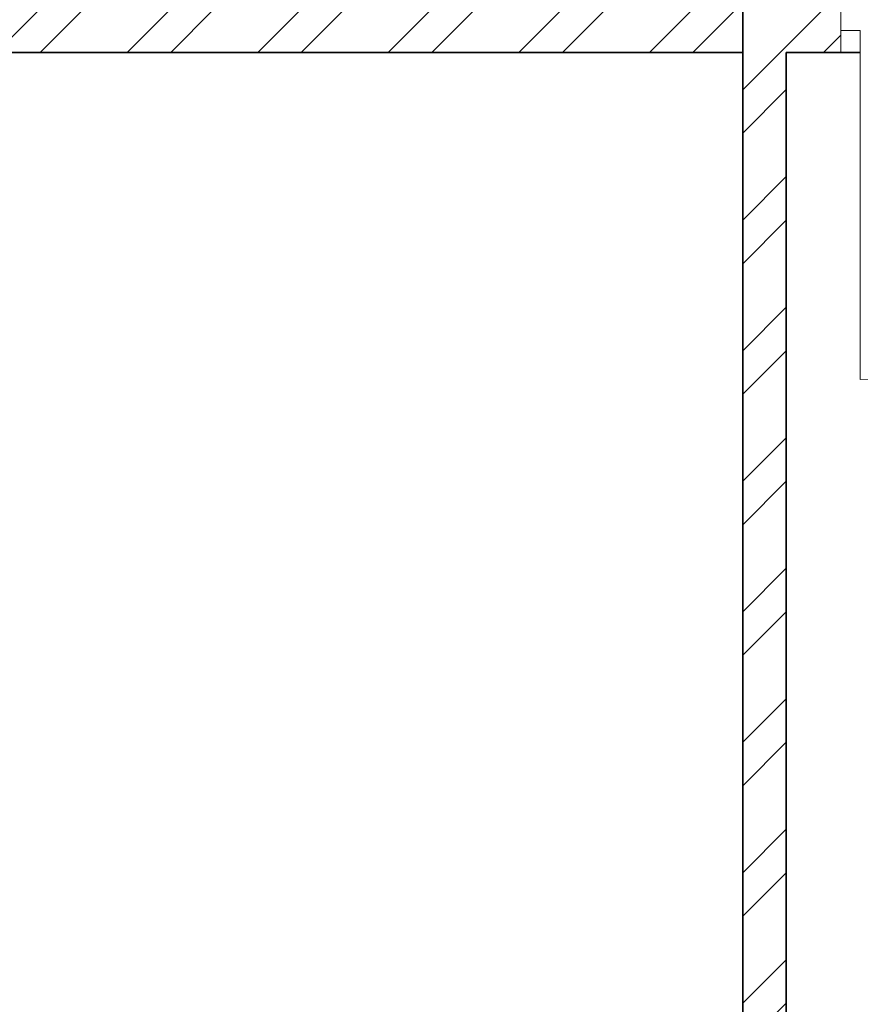
# Model space of a CAD drawing. Units: inches. Extents: x 1962 to 2771, y 1245 to 2660.
# Tile 31 of 114: x 2160 to 2247, y 1831 to 1932. Entities that reach past the tile are written whole.
import ezdxf

# ---------------------------------------------------------------- set-up
doc = ezdxf.new("R2010")
doc.units = ezdxf.units.IN
for name, color, linetype, lineweight in [('A-DOOR', 3, 'Continuous', 18), ('A-WALL', 7, 'Continuous', 35), ('A-WALL-PATT', 252, 'Continuous', 13)]:
    doc.layers.add(name, color=color, linetype=linetype, lineweight=lineweight)

msp = doc.modelspace()

# ---------------------------------------------------------------- hatches: boundary and pattern name
at = {"layer": 'A-WALL-PATT'}
h = msp.add_hatch(dxfattribs=at)
h.set_pattern_fill('ANSI32', color=256)
h.paths.add_polyline_path([(2090.8074, 2467.3437), (2141.6481, 2467.3437), (2141.6481, 2469.5937), (2141.6481, 2471.8437), (2086.3074, 2471.8437), (2086.3074, 2422.5333), (2090.8074, 2422.5333)])
h.paths.add_polyline_path([(2282.7664, 2471.8437), (2204.8982, 2471.8437), (2204.8982, 2467.3437), (2234.8074, 2467.3437), (2234.8074, 2311.3437), (2228.7492, 2311.3437), (2228.7492, 2306.8437), (2234.8074, 2306.8437), (2331.9227, 2306.8437), (2331.9227, 2309.0937), (2331.9227, 2311.3437), (2239.3074, 2311.3437), (2239.3074, 2467.3437), (2282.7664, 2467.3437), (2282.7664, 2469.5937)])
h.paths.add_polyline_path([(2471.4531, 2519.8437), (2552.011, 2519.8437), (2564.3996, 2519.8437), (2564.3996, 2511.1389), (2568.8996, 2511.1389), (2568.8996, 2524.3437), (2466.9531, 2524.3437), (2466.9531, 2471.8437), (2450.0749, 2471.8437), (2446.4672, 2471.8437), (2446.4672, 2467.3437), (2450.0749, 2467.3437), (2475.9988, 2467.3437), (2475.9988, 2469.5937), (2475.9988, 2471.8437), (2471.4531, 2471.8437)])
h.paths.add_polyline_path([(2575.2231, 2469.5937), (2575.2231, 2471.8437), (2568.8996, 2471.8437), (2568.8996, 2487.1389), (2564.3996, 2487.1389), (2564.3996, 2471.8437), (2556.511, 2471.8437), (2499.2904, 2471.8437), (2499.2904, 2467.3437), (2507.8074, 2467.3437), (2507.8074, 2311.3437), (2414.863, 2311.3437), (2414.863, 2306.8437), (2512.3074, 2306.8437), (2517.0114, 2306.8437), (2517.0114, 2309.0937), (2517.0114, 2311.3437), (2512.3074, 2311.3437), (2512.3074, 2467.3437), (2575.2231, 2467.3437)])
h.paths.add_polyline_path([(2660.8074, 2471.8437), (2600.9602, 2471.8437), (2600.9602, 2467.3437), (2656.3074, 2467.3437), (2656.3074, 2432.5704), (2660.8074, 2432.5704)])
h.paths.add_polyline_path([(2660.8074, 2372.5704), (2656.3074, 2372.5704), (2656.3074, 2311.3437), (2600.276, 2311.3437), (2600.276, 2309.0937), (2600.276, 2306.8437), (2656.3074, 2306.8437), (2656.3074, 2296.2593), (2660.8074, 2296.2593)])
h.paths.add_polyline_path([(2572.3074, 2306.8437), (2577.1385, 2306.8437), (2577.1385, 2311.3437), (2551.082, 2311.3437), (2551.082, 2306.8437), (2567.8074, 2306.8437), (2567.8074, 2258.8437), (2540.0574, 2258.8437), (2540.0574, 2256.5937), (2540.0574, 2254.3437), (2567.8074, 2254.3437), (2656.3074, 2254.3437), (2656.3074, 2236.9085), (2660.8074, 2236.9085), (2660.8074, 2272.2593), (2656.3074, 2272.2593), (2656.3074, 2258.8437), (2572.3074, 2258.8437)])
h.paths.add_polyline_path([(2512.3074, 2254.3437), (2518.8716, 2254.3437), (2518.8716, 2256.5937), (2518.8716, 2258.8437), (2507.8074, 2258.8437), (2507.8074, 2177.8437), (2567.8074, 2177.8437), (2567.8074, 2172.9628), (2572.3074, 2172.9628), (2572.3074, 2177.8437), (2656.3074, 2177.8437), (2656.3074, 2166.4846), (2660.8074, 2166.4846), (2660.8074, 2200.9085), (2656.3074, 2200.9085), (2656.3074, 2182.3437), (2512.3074, 2182.3437)])
h.paths.add_polyline_path([(2656.3074, 2129.8437), (2572.3074, 2129.8437), (2572.3074, 2150.3044), (2570.0574, 2150.3044), (2567.8074, 2150.3044), (2567.8074, 2129.8437), (2507.8074, 2129.8437), (2507.8074, 2116.3027), (2510.0574, 2116.3027), (2512.3074, 2116.3027), (2512.3074, 2125.3437), (2567.8074, 2125.3437), (2572.3074, 2125.3437), (2656.3074, 2125.3437)])
h.paths.add_polyline_path([(2090.8074, 2362.5333), (2086.3074, 2362.5333), (2086.3074, 2298.6242), (2090.8074, 2298.6242), (2090.8074, 2306.8437), (2174.8074, 2306.8437), (2174.8074, 2286.4178), (2179.3074, 2286.4178), (2179.3074, 2306.8437), (2192.8641, 2306.8437), (2192.8641, 2309.0937), (2192.8641, 2311.3437), (2090.8074, 2311.3437)])
h.paths.add_polyline_path([(2209.156, 2258.8437), (2179.3074, 2258.8437), (2179.3074, 2263.2236), (2177.0574, 2263.2236), (2174.8074, 2263.2236), (2174.8074, 2258.8437), (2090.8074, 2258.8437), (2090.8074, 2274.6242), (2086.3074, 2274.6242), (2086.3074, 2238.2967), (2088.5574, 2238.2967), (2090.8074, 2238.2967), (2090.8074, 2254.3437), (2209.156, 2254.3437)])
h.paths.add_polyline_path([(2090.8074, 2177.8437), (2234.8074, 2177.8437), (2234.8074, 2173.1428), (2239.3074, 2173.1428), (2239.3074, 2258.8437), (2230.8442, 2258.8437), (2230.8442, 2256.5937), (2230.8442, 2254.3437), (2234.8074, 2254.3437), (2234.8074, 2182.3437), (2090.8074, 2182.3437), (2090.8074, 2202.2967), (2086.3074, 2202.2967), (2086.3074, 2140.0389), (2090.8074, 2140.0389)])
h.paths.add_polyline_path([(2090.8074, 2080.0389), (2086.3074, 2080.0389), (2086.3074, 2033.8437), (2090.8074, 2033.8437)], flags=17)
h.paths.add_polyline_path([(2244.9405, 2033.8437), (2239.3074, 2033.8437), (2239.3074, 2142.0665), (2237.2592, 2142.0665), (2234.8074, 2142.0665), (2234.8074, 2033.8437), (2090.8074, 2033.8437), (2076.5204, 2033.8437), (2072.0204, 2033.8437), (2072.0204, 2000.4493), (2076.5204, 2000.4493), (2076.5204, 2029.3437), (2090.8074, 2029.3437), (2244.9405, 2029.3437), (2244.9405, 2031.5937)])
h.paths.add_polyline_path([(2234.8074, 1933.3437), (2076.5204, 1933.3437), (2076.5204, 1952.4493), (2074.2704, 1952.4493), (2072.0204, 1952.4493), (2072.0204, 1933.3437), (2072.0204, 1928.8437), (2234.8074, 1928.8437)])
h.paths.add_polyline_path([(2090.8074, 1928.8437), (2086.3074, 1928.8437), (2086.3074, 1906.5013), (2090.8074, 1906.5013)])
h.paths.add_polyline_path([(2090.8074, 1846.5013), (2086.3074, 1846.5013), (2086.3074, 1769.9917), (2088.5574, 1769.9917), (2090.8074, 1769.9917), (2090.8074, 1780.3437), (2234.8074, 1780.3437), (2234.8074, 1708.3437), (2230.3764, 1708.3437), (2230.3764, 1703.8437), (2239.3074, 1703.8437), (2239.3074, 1792.6669), (2237.0574, 1792.6669), (2234.8074, 1792.6669), (2234.8074, 1784.8437), (2090.8074, 1784.8437)])
h.paths.add_polyline_path([(2239.3074, 1928.8437), (2244.9405, 1928.8437), (2244.9405, 1931.0937), (2244.9405, 1933.3437), (2234.8074, 1933.3437), (2234.8074, 1928.8437), (2234.8074, 1825.5949), (2239.3074, 1825.5949)])
h.paths.add_polyline_path([(2148.0425, 1649.0937), (2148.0425, 1651.3437), (2090.8074, 1651.3437), (2090.8074, 1646.8437), (2148.0425, 1646.8437)], flags=0)
h.paths.add_polyline_path([(2207.5601, 1708.3437), (2090.8074, 1708.3437), (2090.8074, 1703.8437), (2174.8074, 1703.8437), (2174.8074, 1651.3437), (2170.4457, 1651.3437), (2170.4457, 1646.8437), (2195.9924, 1646.8437), (2195.9924, 1649.0937), (2195.9924, 1651.3437), (2179.3074, 1651.3437), (2179.3074, 1703.8437), (2207.5601, 1703.8437), (2207.5601, 1706.0937)])
h.paths.add_polyline_path([(2090.8074, 1733.9917), (2086.3074, 1733.9917), (2086.3074, 1696.1032), (2088.5574, 1696.1032), (2090.8074, 1696.1032)])
h.paths.add_polyline_path([(2090.8074, 1672.1032), (2086.3074, 1672.1032), (2086.3074, 1600.3335), (2090.8074, 1600.3335)])
h.paths.add_polyline_path([(2090.8074, 1540.3335), (2086.3074, 1540.3335), (2086.3074, 1486.3437), (2139.6766, 1486.3437), (2139.6766, 1490.8437), (2090.8074, 1490.8437)])
h.paths.add_polyline_path([(2302.3876, 1490.8437), (2239.3074, 1490.8437), (2239.3074, 1646.8437), (2335.9994, 1646.8437), (2335.9994, 1651.3437), (2229.884, 1651.3437), (2229.884, 1646.8437), (2234.8074, 1646.8437), (2234.8074, 1490.8437), (2202.7103, 1490.8437), (2202.7103, 1488.5937), (2202.7103, 1486.3437), (2275.0699, 1486.3437), (2275.0699, 1475.772), (2279.5699, 1475.772), (2279.5699, 1486.3437), (2302.3876, 1486.3437)])
h.paths.add_polyline_path([(2279.5699, 1451.772), (2275.0699, 1451.772), (2275.0699, 1438.3437), (2174.8074, 1438.3437), (2174.8074, 1486.3437), (2179.7922, 1486.3437), (2179.7922, 1490.8437), (2163.3585, 1490.8437), (2163.3585, 1488.5937), (2163.3585, 1486.3437), (2170.3074, 1486.3437), (2170.3074, 1433.8437), (2279.5699, 1433.8437)])
h.paths.add_polyline_path([(2427.2363, 1490.8437), (2375.8074, 1490.8437), (2375.8074, 1646.8437), (2381.6401, 1646.8437), (2381.6401, 1651.3437), (2365.887, 1651.3437), (2365.887, 1649.0937), (2365.887, 1646.8437), (2371.3074, 1646.8437), (2371.3074, 1490.8437), (2327.5627, 1490.8437), (2327.5627, 1488.5937), (2327.5627, 1486.3437), (2371.3074, 1486.3437), (2371.3074, 1433.8437), (2375.8074, 1433.8437), (2375.8074, 1486.3437), (2427.2363, 1486.3437)])
h.paths.add_polyline_path([(2512.3074, 1646.8437), (2519.4351, 1646.8437), (2519.4351, 1649.0937), (2519.4351, 1651.3437), (2507.8074, 1651.3437), (2416.0063, 1651.3437), (2416.0063, 1649.0937), (2416.0063, 1646.8437), (2507.8074, 1646.8437), (2507.8074, 1490.8437), (2497.0532, 1490.8437), (2497.0532, 1488.5937), (2497.0532, 1486.3437), (2574.9344, 1486.3437), (2574.9344, 1476.0181), (2579.4344, 1476.0181), (2579.4344, 1486.3437), (2584.4872, 1486.3437), (2584.3074, 1490.8437), (2512.3074, 1490.8437)])
h.paths.add_polyline_path([(2470.5091, 1486.3437), (2473.9767, 1486.3437), (2473.9767, 1490.8437), (2449.6605, 1490.8437), (2449.6605, 1488.5937), (2449.6605, 1486.3437), (2466.0091, 1486.3437), (2466.0091, 1433.8437), (2470.5091, 1433.8437), (2579.4344, 1433.8437), (2579.4344, 1452.0181), (2574.9344, 1452.0181), (2574.9344, 1438.3437), (2554.5091, 1438.3437), (2470.5091, 1438.3437)])
h.paths.add_polyline_path([(2656.3074, 1490.8437), (2611.86, 1490.8437), (2611.86, 1486.3437), (2656.3074, 1486.3437)])
h.paths.add_polyline_path([(2660.8074, 1532.7007), (2658.5574, 1532.7007), (2656.3074, 1532.7007), (2656.3074, 1486.3437), (2660.8074, 1486.3437)])
h.paths.add_polyline_path([(2660.8074, 1664.9663), (2656.3074, 1664.9663), (2656.3074, 1651.3437), (2602.2313, 1651.3437), (2602.2313, 1646.8437), (2656.3074, 1646.8437), (2656.3074, 1592.7007), (2660.8074, 1592.7007)])
h.paths.add_polyline_path([(2660.8074, 1724.5221), (2656.3074, 1724.5221), (2656.3074, 1703.8437), (2542.4725, 1703.8437), (2542.4725, 1699.3437), (2567.8074, 1699.3437), (2567.8074, 1651.3437), (2552.7766, 1651.3437), (2552.7766, 1649.0937), (2552.7766, 1646.8437), (2577.2878, 1646.8437), (2577.2878, 1649.0937), (2577.2878, 1651.3437), (2572.3074, 1651.3437), (2572.3074, 1699.3437), (2656.3074, 1699.3437), (2656.3074, 1688.9663), (2660.8074, 1688.9663)])
h.paths.add_polyline_path([(2660.8074, 1880.6524), (2656.3074, 1880.6524), (2656.3074, 1832.8437), (2512.3074, 1832.8437), (2512.3074, 1837.8959), (2507.8074, 1837.8959), (2507.8074, 1828.3437), (2567.8074, 1828.3437), (2567.8074, 1804.3437), (2572.3074, 1804.3437), (2572.3074, 1828.3437), (2656.3074, 1828.3437), (2656.3074, 1818.6778), (2660.8074, 1818.6778)])
h.paths.add_polyline_path([(2660.8074, 1794.6778), (2656.3074, 1794.6778), (2656.3074, 1780.3437), (2572.3074, 1780.3437), (2572.3074, 1783.0303), (2570.0574, 1783.0303), (2567.8074, 1783.0303), (2567.8074, 1780.3437), (2507.8074, 1780.3437), (2507.8074, 1699.3437), (2517.8858, 1699.3437), (2517.8858, 1701.5937), (2517.8858, 1703.8437), (2512.3074, 1703.8437), (2512.3074, 1775.8437), (2656.3074, 1775.8437), (2656.3074, 1760.5221), (2660.8074, 1760.5221)])
h.paths.add_polyline_path([(2660.8074, 1981.3437), (2660.8074, 2020.2808), (2658.5574, 2020.2808), (2656.3074, 2020.2808), (2656.3074, 1981.3437), (2512.3074, 1981.3437), (2512.3074, 2086.6996), (2507.8074, 2086.6996), (2507.8074, 1981.3437), (2375.8074, 1981.3437), (2375.8074, 1986.8505), (2373.5574, 1986.8505), (2371.3074, 1986.8505), (2371.3074, 1973.2607), (2375.8074, 1973.2607), (2375.8074, 1976.8437), (2507.8074, 1976.8437), (2507.8074, 1865.4281), (2510.0574, 1865.4281), (2512.3074, 1865.4281), (2512.3074, 1976.8437), (2660.8074, 1976.8437)])
h.paths.add_polyline_path([(2375.8074, 1940.297), (2373.5574, 1940.297), (2371.3074, 1940.297), (2371.3074, 1933.3437), (2278.4434, 1933.3437), (2278.4434, 1928.8437), (2371.3074, 1928.8437), (2371.3074, 1651.3437), (2375.8074, 1651.3437)])
h.paths.add_polyline_path([(2660.8074, 1976.8437), (2656.3074, 1976.8437), (2656.3074, 1940.6524), (2660.8074, 1940.6524)], flags=17)
h.paths.add_polyline_path([(2660.8074, 2142.4846), (2656.3074, 2142.4846), (2656.3074, 2080.2808), (2660.8074, 2080.2808)])
h.paths.add_polyline_path([(2381.4189, 2311.3437), (2375.8074, 2311.3437), (2375.8074, 2467.3437), (2424.7242, 2467.3437), (2424.7242, 2469.5937), (2424.7242, 2471.8437), (2375.8074, 2471.8437), (2375.8074, 2524.3437), (2371.3074, 2524.3437), (2371.3074, 2471.8437), (2307.2097, 2471.8437), (2307.2097, 2467.3437), (2371.3074, 2467.3437), (2371.3074, 2311.3437), (2366.8901, 2311.3437), (2366.8901, 2306.8437), (2371.3074, 2306.8437), (2371.3074, 2033.8437), (2279.6589, 2033.8437), (2279.6589, 2029.3437), (2371.3074, 2029.3437), (2371.3074, 2014.2598), (2375.8074, 2014.2598), (2375.8074, 2306.8437), (2381.4189, 2306.8437)])
h.paths.add_polyline_path([(2263.3074, 2524.3437), (2170.3074, 2524.3437), (2170.3074, 2519.8437), (2170.3074, 2471.8437), (2165.0312, 2471.8437), (2165.0312, 2467.3437), (2179.6721, 2467.3437), (2179.6721, 2469.5161), (2179.6721, 2471.8437), (2174.8074, 2471.8437), (2174.8074, 2519.8437), (2258.8074, 2519.8437), (2258.8074, 2511.6436), (2263.3074, 2511.6436)])
h.paths.add_polyline_path([(2245.0232, 1361.4123), (2492.9468, 1361.4123), (2492.9468, 1398.505), (2245.0232, 1398.505)], flags=9)
h.paths.add_polyline_path([(2388.1434, 2086.6936), (2425.0704, 2086.6936), (2425.0704, 2105.3509), (2388.1434, 2105.3509)], flags=9)
h.paths.add_polyline_path([(2404.922, 2242.6744), (2445.7337, 2242.6744), (2445.7337, 2261.3318), (2404.922, 2261.3318)], flags=9)
h.paths.add_polyline_path([(2269.4107, 2156.7935), (2306.3378, 2156.7935), (2306.3378, 2175.4508), (2269.4107, 2175.4508)], flags=9)
h.paths.add_polyline_path([(2269.3277, 2233.4343), (2306.2547, 2233.4343), (2306.2547, 2252.0917), (2269.3277, 2252.0917)], flags=9)
h.paths.add_polyline_path([(2431.6052, 2320.6922), (2470.4456, 2320.6922), (2470.4456, 2339.3495), (2431.6052, 2339.3495)], flags=25)
h.paths.add_polyline_path([(2249.6902, 2315.7608), (2288.5306, 2315.7608), (2288.5306, 2334.4182), (2249.6902, 2334.4182)], flags=25)
h.paths.add_polyline_path([(2096.9301, 2314.3181), (2135.7704, 2314.3181), (2135.7704, 2332.9755), (2096.9301, 2332.9755)], flags=25)
h.paths.add_polyline_path([(2134.3475, 2285.7089), (2161.4655, 2285.7089), (2161.4655, 2304.3662), (2134.3475, 2304.3662)], flags=9)
h.paths.add_polyline_path([(2126.5155, 2209.4076), (2159.9227, 2209.4076), (2159.9227, 2228.065), (2126.5155, 2228.065)], flags=25)
h.paths.add_polyline_path([(2110.5753, 2141.5299), (2149.4157, 2141.5299), (2149.4157, 2160.1872), (2110.5753, 2160.1872)], flags=25)
h.paths.add_polyline_path([(2249.8618, 1968.3317), (2286.3966, 1968.3317), (2286.3966, 1986.989), (2249.8618, 1986.989)], flags=9)
h.paths.add_polyline_path([(2395.9507, 1777.0051), (2436.7624, 1777.0051), (2436.7624, 1795.6625), (2395.9507, 1795.6625)], flags=9)
h.paths.add_polyline_path([(2398.5259, 1888.5651), (2435.0062, 1888.5651), (2435.0062, 1907.2224), (2398.5259, 1907.2224)], flags=25)
h.paths.add_polyline_path([(2259.3506, 1728.3559), (2296.2776, 1728.3559), (2296.2776, 1747.0132), (2259.3506, 1747.0132)], flags=9)
h.paths.add_polyline_path([(2271.3698, 1845.268), (2308.2968, 1845.268), (2308.2968, 1863.9253), (2271.3698, 1863.9253)], flags=9)
h.paths.add_polyline_path([(2120.9355, 1786.3027), (2159.7759, 1786.3027), (2159.7759, 1804.9601), (2120.9355, 1804.9601)], flags=25)
h.paths.add_polyline_path([(2121.3164, 1732.1043), (2154.7236, 1732.1043), (2154.7236, 1750.7616), (2121.3164, 1750.7616)], flags=25)
h.paths.add_polyline_path([(2118.3706, 1678.8997), (2147.5282, 1678.8997), (2147.5282, 1697.557), (2118.3706, 1697.557)], flags=25)
h.paths.add_polyline_path([(2385.9227, 1493.557), (2424.763, 1493.557), (2424.763, 1512.2143), (2385.9227, 1512.2143)], flags=25)
h.paths.add_polyline_path([(2248.7058, 1500.0256), (2287.5462, 1500.0256), (2287.5462, 1518.6829), (2248.7058, 1518.6829)], flags=25)
h.paths.add_polyline_path([(2104.1669, 1617.3771), (2143.0073, 1617.3771), (2143.0073, 1636.0344), (2104.1669, 1636.0344)], flags=9)
h.paths.add_polyline_path([(2096.0714, 1447.8824), (2137.3845, 1447.8824), (2137.3845, 1458.1859), (2096.0714, 1458.1859)], flags=9)
h.paths.add_polyline_path([(2180.6114, 1440.325), (2209.7689, 1440.325), (2209.7689, 1458.9823), (2180.6114, 1458.9823)], flags=25)
h.paths.add_polyline_path([(2316.1698, 1447.9637), (2357.4829, 1447.9637), (2357.4829, 1458.2673), (2316.1698, 1458.2673)], flags=9)
h.paths.add_polyline_path([(2397.6187, 1447.9637), (2438.9318, 1447.9637), (2438.9318, 1458.2673), (2397.6187, 1458.2673)], flags=9)
h.paths.add_polyline_path([(2473.0778, 1439.5953), (2502.2354, 1439.5953), (2502.2354, 1458.2527), (2473.0778, 1458.2527)], flags=25)
h.paths.add_polyline_path([(2589.7027, 1447.8819), (2631.0158, 1447.8819), (2631.0158, 1458.1855), (2589.7027, 1458.1855)], flags=9)
h.paths.add_polyline_path([(2522.4009, 1497.5285), (2561.2413, 1497.5285), (2561.2413, 1516.1859), (2522.4009, 1516.1859)], flags=25)
h.paths.add_polyline_path([(2579.6565, 1671.3482), (2608.8141, 1671.3482), (2608.8141, 1690.0056), (2579.6565, 1690.0056)], flags=25)
h.paths.add_polyline_path([(2544.7038, 1725.5064), (2578.1111, 1725.5064), (2578.1111, 1744.1637), (2544.7038, 1744.1637)], flags=25)
h.paths.add_polyline_path([(2578.1191, 1807.472), (2607.2766, 1807.472), (2607.2766, 1826.1293), (2578.1191, 1826.1293)], flags=25)
h.paths.add_polyline_path([(2595.0614, 1835.1839), (2633.9018, 1835.1839), (2633.9018, 1853.8413), (2595.0614, 1853.8413)], flags=25)
h.paths.add_polyline_path([(2567.0097, 2097.7035), (2605.8501, 2097.7035), (2605.8501, 2116.3609), (2567.0097, 2116.3609)], flags=9)
h.paths.add_polyline_path([(2586.644, 2134.6454), (2615.8015, 2134.6454), (2615.8015, 2153.3027), (2586.644, 2153.3027)], flags=9)
h.paths.add_polyline_path([(2544.6185, 2212.6783), (2578.0258, 2212.6783), (2578.0258, 2231.3356), (2544.6185, 2231.3356)], flags=25)
h.paths.add_polyline_path([(2577.0273, 2256.9023), (2606.1849, 2256.9023), (2606.1849, 2275.5597), (2577.0273, 2275.5597)], flags=24)
h.paths.add_polyline_path([(2605.2683, 2315.2821), (2644.1087, 2315.2821), (2644.1087, 2333.9395), (2605.2683, 2333.9395)], flags=25)
h.paths.add_polyline_path([(2583.1244, 2496.1815), (2624.4375, 2496.1815), (2624.4375, 2506.4851), (2583.1244, 2506.4851)], flags=9)
h.paths.add_polyline_path([(2474.761, 2497.0823), (2503.9185, 2497.0823), (2503.9185, 2515.7397), (2474.761, 2515.7397)], flags=25)
h.paths.add_polyline_path([(2387.5787, 2494.2563), (2428.902, 2494.2563), (2428.902, 2504.5598), (2387.5787, 2504.5598)], flags=9)
h.paths.add_polyline_path([(2300.1657, 2500.1564), (2341.4788, 2500.1564), (2341.4788, 2510.46), (2300.1657, 2510.46)], flags=25)
h.paths.add_polyline_path([(2176.8589, 2497.5843), (2206.0165, 2497.5843), (2206.0165, 2516.2416), (2176.8589, 2516.2416)], flags=25)
h.paths.add_polyline_path([(2097.4668, 2494.9762), (2138.7799, 2494.9762), (2138.7799, 2505.2798), (2097.4668, 2505.2798)], flags=9)

# ---------------------------------------------------------------- linework, layer by layer
at = {"layer": 'A-DOOR'}
for p, q in [((2244.9405, 1933.3437), (2244.9405, 1928.8437)), ((2244.9405, 1928.8437), (2244.9405, 1931.0937)), ((2244.9405, 1931.0937), (2246.9405, 1931.0937)), ((2246.9405, 1931.0937), (2246.9405, 1895.0937))]:
    msp.add_line(p, q, dxfattribs=at)
msp.add_arc((2246.9405, 1925.1829), 30.0892, 270, 11.329108, dxfattribs=at)
at = {"layer": 'A-WALL'}
for p, q in [((2234.8074, 1933.3437), (2234.8074, 1824.0006)), ((2072.0204, 1928.8437), (2234.8074, 1928.8437)), ((2239.3074, 1928.8437), (2239.3074, 1825.5949)), ((2239.3074, 1928.8437), (2246.9405, 1928.8437))]:
    msp.add_line(p, q, dxfattribs=at)

doc.saveas('drawing.dxf')
